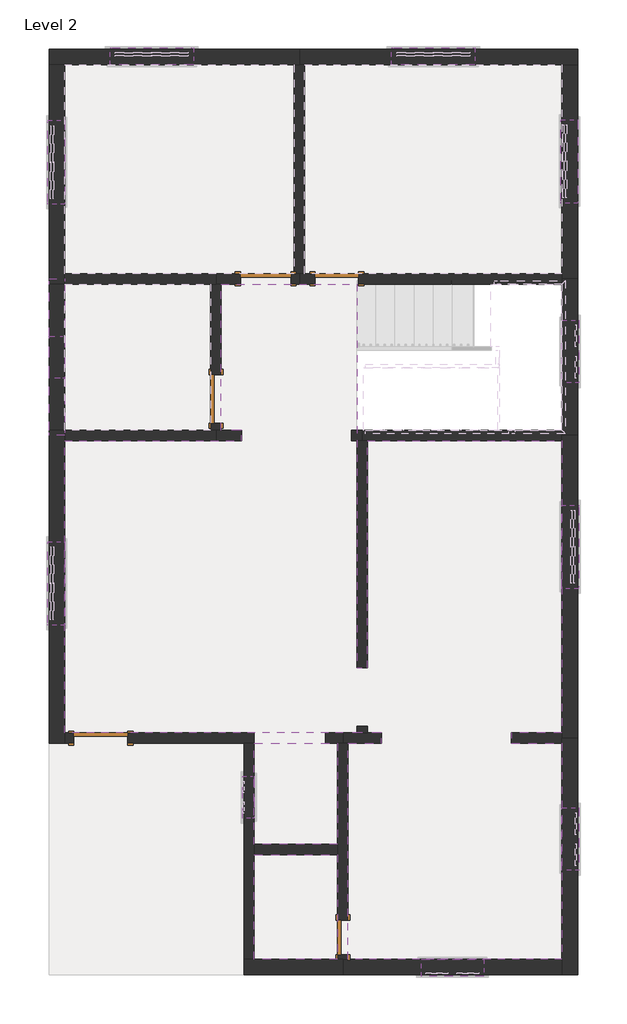
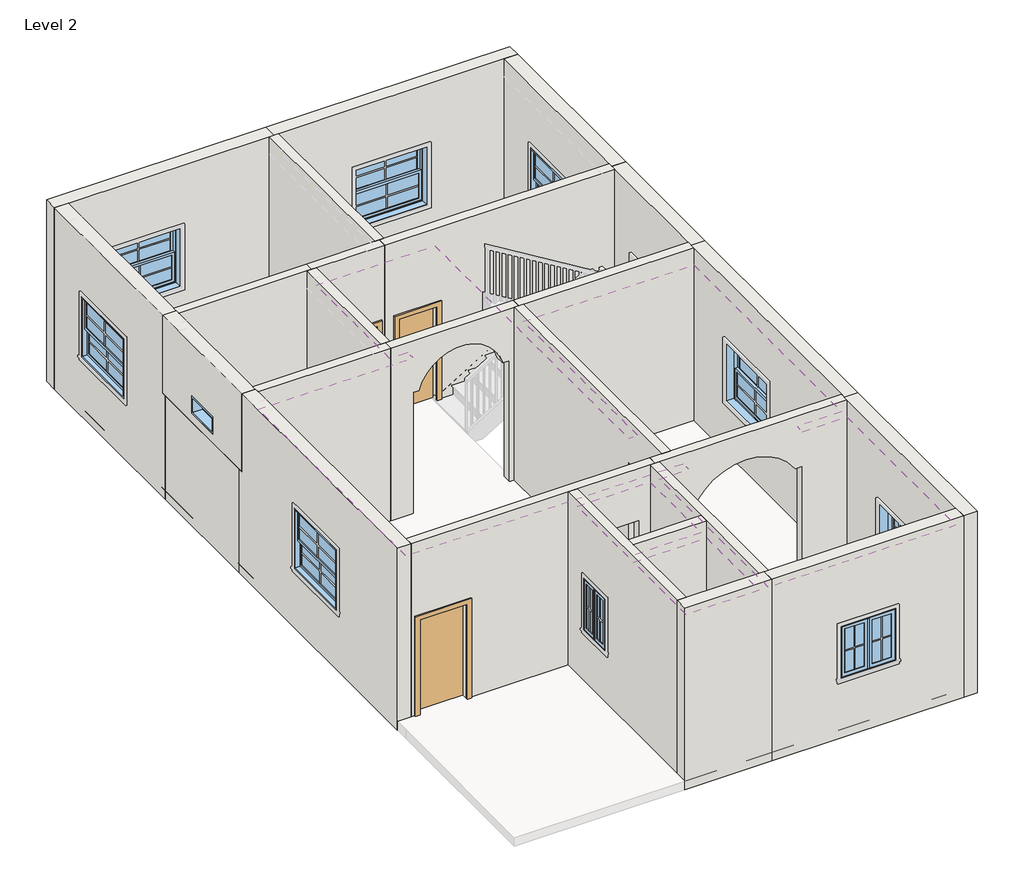
# One storey, part 1 of 2: 26 walls, 11 windows, 5 doors, 3 coverings.
"""IFC4 building model written with IfcOpenShell, lengths in millimetres."""

from ifc_helpers import new_model, si_unit, frame, origin, place, context, project, spatial, polyline, circle_curve, outline, extrude, faceted_brep, transform, mapped, element, save
from ifc_brep_helpers import plane_surface, revolved_surface, advanced_brep
from components import door_85c31a06, door_fe267433, door_77f51d0b, door_a6948854, door_ee35e093, fixed_2_8c8825d0, window_casement_double_2_fb285ced, window_casement_double_3_90de19e9, window_double_hung_4_eadb0177, window_double_hung_4_aab3aae7

model = new_model("IFC4")

# Units and contexts
model_context = context("Model", 3, world=origin())
ifc_project = project(units=[si_unit("LENGTHUNIT", "METRE", prefix="MILLI")], contexts=[model_context])

# Site, building, storey
site = spatial("IfcSite", under=ifc_project)
building = spatial("IfcBuilding", under=site)
storey = spatial("IfcBuildingStorey", under=building, Name="Level 2", Elevation=3200.4)

# Coverings
placement = place(None, origin())
element("IfcCovering", 1, ObjectType="2' x 4' ACT System", at=placement, inside=storey, context=model_context, shape_type="SweptSolid", body=[
    extrude(outline(polyline([(1592.635938, -3451.4142637), (1592.635938, -6601.0142637), (-1531.564062, -6601.0142637), (-1531.564062, -3451.4142637), (-1042.9877715, -3451.4142637), (-1042.9877715, -3299.0142637), (-1607.764062, -3299.0142637), (-5671.764062, -3299.0142637), (-5671.764062, 968.1857363), (-3538.164062, 968.1857363), (-3088.5741654, 968.1857363), (-3088.5741654, 1120.5857363), (-3385.764062, 1120.5857363), (-3385.764062, 3254.1857363), (-2242.764062, 3254.1857363), (-1404.564062, 3254.1857363), (-1404.564062, -2346.4297845), (-1252.164062, -2346.4297845), (-1252.164062, 968.1857363), (1592.635938, 968.1857363), (1592.635938, -3299.0142637), (852.655246, -3299.0142637), (852.655246, -3451.4142637), (1592.635938, -3451.4142637)])), frame((0.0, 0.0, 6248.4), z_axis=(0.0, 0.0, 1.0), x_axis=(1.0, 0.0, 0.0)), (0.0, 0.0, 1.0), 57.15),
])
element("IfcCovering", 2, ObjectType="2' x 4' ACT System", at=placement, inside=storey, context=model_context, shape_type="SweptSolid", body=[
    extrude(outline(polyline([(-2903.164062, -4924.6142637), (-2903.164062, -3451.4142637), (-1683.964062, -3451.4142637), (-1683.964062, -4924.6142637), (-2903.164062, -4924.6142637)])), frame((0.0, 0.0, 6248.4), z_axis=(0.0, 0.0, 1.0), x_axis=(1.0, 0.0, 0.0)), (0.0, 0.0, 1.0), 57.15),
])
element("IfcCovering", 3, ObjectType="2' x 4' ACT System", at=placement, inside=storey, context=model_context, shape_type="SweptSolid", body=[
    extrude(outline(polyline([(-2903.164062, -6601.0142637), (-2903.164062, -5077.0142637), (-1683.964062, -5077.0142637), (-1683.964062, -6601.0142637), (-2903.164062, -6601.0142637)])), frame((0.0, 0.0, 6248.4), z_axis=(0.0, 0.0, 1.0), x_axis=(1.0, 0.0, 0.0)), (0.0, 0.0, 1.0), 57.15),
])

# Doors
door_shape = door_85c31a06(model_context)
element("IfcDoor", 4, ObjectType="Single-Flush : 1'8\"", at=placement, inside=storey, context=model_context, shape_type="MappedRepresentation", body=[
    mapped(door_shape, transform((-1607.764062, -6283.5142637, 3352.8), x_axis=(0.0, -1.0, 0.0), y_axis=(1.0, 0.0, 0.0), z_axis=(0.0, 0.0, 1.0))),
])
door_2_shape = door_fe267433(model_context)
element("IfcDoor", 5, ObjectType="Single-Flush : 2'1\"", at=placement, inside=storey, context=model_context, shape_type="MappedRepresentation", body=[
    mapped(door_2_shape, transform((-1696.664062, 3330.3857363, 3352.8), x_axis=(-1.0, 0.0, 0.0), y_axis=(0.0, -1.0, 0.0), z_axis=(0.0, 0.0, 1.0))),
])
door_3_shape = door_77f51d0b(model_context)
element("IfcDoor", 6, ObjectType="Single-Flush : 2'4\"", at=placement, inside=storey, context=model_context, shape_type="MappedRepresentation", body=[
    mapped(door_3_shape, transform((-3461.964062, 1577.7857363, 3352.8), x_axis=(0.0, -1.0, 0.0), y_axis=(1.0, 0.0, 0.0), z_axis=(0.0, 0.0, 1.0))),
])
door_4_shape = door_a6948854(model_context)
element("IfcDoor", 7, ObjectType="Single-Flush : 2'5\"", at=placement, inside=storey, context=model_context, shape_type="MappedRepresentation", body=[
    mapped(door_4_shape, transform((-2738.064062, 3330.3857363, 3352.8), x_axis=(1.0, 0.0, 0.0), y_axis=(0.0, 1.0, 0.0), z_axis=(0.0, 0.0, 1.0))),
])
door_5_shape = door_ee35e093(model_context)
element("IfcDoor", 8, ObjectType="Single-Flush : 2'7\"", at=placement, inside=storey, context=model_context, shape_type="MappedRepresentation", body=[
    mapped(door_5_shape, transform((-5144.714062, -3375.2142637, 3352.8), x_axis=(-1.0, 0.0, 0.0), y_axis=(0.0, -1.0, 0.0), z_axis=(0.0, 0.0, 1.0))),
])

# Walls
element("IfcWall", 9, ObjectType="Generic - 6\"", at=placement, inside=storey, context=model_context, shape_type="Brep", body=[
    faceted_brep([(-2318.964062, 6454.5857363, 3352.8), (-2318.964062, 3406.5857363, 3352.8), (-2318.964062, 3406.5857363, 6553.2), (-2318.964062, 6454.5857363, 6553.2), (-2166.564062, 6454.5857363, 3352.8), (-2166.564062, 6454.5857363, 6553.2), (-2166.564062, 3406.5857363, 6553.2), (-2166.564062, 3406.5857363, 3352.8), (-2242.764062, 6454.5857363, 3352.8), (-2242.764062, 3406.5857363, 3352.8), (-2242.764062, 3406.5857363, 6553.2), (-2242.764062, 6454.5857363, 6553.2)], [[[0, 1, 2, 3]], [[4, 5, 6, 7]], [[1, 0, 8, 4, 7, 9]], [[3, 2, 10, 6, 5, 11]], [[0, 3, 11, 5, 4, 8]], [[2, 1, 9, 7, 6, 10]]]),
])
element("IfcWall", 10, ObjectType="Generic - 6\"", at=placement, inside=storey, context=model_context, shape_type="Brep", body=[
    faceted_brep([(-5671.764062, 3254.1857363, 6553.2), (-5671.764062, 3254.1857363, 5181.6), (-5671.764062, 3254.1857363, 3352.8), (-3538.164062, 3254.1857363, 3352.8), (-3461.964062, 3254.1857363, 3352.8), (-3461.964062, 3254.1857363, 6553.2), (-3538.164062, 3254.1857363, 6553.2), (-5671.764062, 3406.5857363, 3352.8), (-5671.764062, 3406.5857363, 6553.2), (-3461.964062, 3406.5857363, 6553.2), (-3461.964062, 3406.5857363, 3352.8), (-5671.764062, 3330.3857363, 6553.2)], [[[0, 1, 2, 3, 4, 5, 6]], [[7, 8, 9, 10]], [[4, 3, 2, 7, 10]], [[5, 4, 10, 9]], [[0, 6, 5, 9, 8, 11]], [[0, 11, 8, 7, 2, 1]]]),
])
element("IfcWall", 11, ObjectType="Generic - 6\"", at=placement, inside=storey, context=model_context, shape_type="Brep", body=[
    faceted_brep([(-5671.764062, 968.1857363, 6553.2), (-5671.764062, 968.1857363, 3352.8), (-3461.964062, 968.1857363, 3352.8), (-3461.964062, 968.1857363, 6553.2), (-5671.764062, 1120.5857363, 3352.8), (-5671.764062, 1120.5857363, 5181.6), (-5671.764062, 1120.5857363, 6553.2), (-3538.164062, 1120.5857363, 6553.2), (-3461.964062, 1120.5857363, 6553.2), (-3461.964062, 1120.5857363, 3352.8), (-3538.164062, 1120.5857363, 3352.8), (-5671.764062, 1044.3857363, 6553.2)], [[[0, 1, 2, 3]], [[4, 5, 6, 7, 8, 9, 10]], [[2, 1, 4, 10, 9]], [[3, 2, 9, 8]], [[0, 3, 8, 7, 6, 11]], [[0, 11, 6, 5, 4, 1]]]),
])
element("IfcWall", 12, ObjectType="Generic - 6\"", at=placement, inside=storey, context=model_context, shape_type="Brep", body=[
    faceted_brep([(-1404.564062, 968.1857363, 3352.8), (-1404.564062, -2346.4297845, 3352.8), (-1404.564062, -2346.4297845, 5816.6), (-1404.564062, -3197.4142637, 5816.6), (-1404.564062, -3197.4142637, 5638.8), (-1404.564062, -3197.4142637, 3352.8), (-1404.564062, -3299.0142637, 3352.8), (-1404.564062, -3299.0142637, 6553.2), (-1404.564062, 968.1857363, 6553.2), (-1252.164062, -2346.4297845, 3352.8), (-1252.164062, 968.1857363, 3352.8), (-1252.164062, 968.1857363, 6553.2), (-1252.164062, -3299.0142637, 6553.2), (-1252.164062, -3299.0142637, 3352.8), (-1252.164062, -3197.4142637, 3352.8), (-1252.164062, -3197.4142637, 5638.8), (-1252.164062, -3197.4142637, 5816.6), (-1252.164062, -2346.4297845, 5816.6), (-1328.364062, 968.1857363, 3352.8), (-1328.364062, 968.1857363, 6553.2)], [[[0, 1, 2, 3, 4, 5, 6, 7, 8]], [[9, 10, 11, 12, 13, 14, 15, 16, 17]], [[7, 6, 13, 12]], [[1, 0, 18, 10, 9]], [[8, 7, 12, 11, 19]], [[2, 1, 9, 17]], [[3, 2, 17, 16]], [[3, 16, 15, 14, 5, 4]], [[6, 5, 14, 13]], [[0, 8, 19, 11, 10, 18]]]),
])
element("IfcWall", 13, ObjectType="Generic - 6\"", at=placement, inside=storey, context=model_context, shape_type="Brep", body=[
    faceted_brep([(-2903.164062, -3451.4142637, 5638.8), (-1865.8319448, -3451.4142637, 5638.8), (-1865.8319448, -3451.4142637, 3352.8), (-1683.964062, -3451.4142637, 3352.8), (-1607.764062, -3451.4142637, 3352.8), (-1607.764062, -3451.4142637, 6553.2), (-1683.964062, -3451.4142637, 6553.2), (-2903.164062, -3451.4142637, 6553.2), (-3055.564062, -3451.4142637, 6553.2), (-5671.764062, -3451.4142637, 6553.2), (-5671.764062, -3451.4142637, 3352.8), (-5538.414062, -3451.4142637, 3352.8), (-5538.414062, -3451.4142637, 5181.6), (-4751.014062, -3451.4142637, 5181.6), (-4751.014062, -3451.4142637, 3352.8), (-3055.564062, -3451.4142637, 3352.8), (-2903.164062, -3451.4142637, 3352.8), (-1865.8319448, -3299.0142637, 5638.8), (-2903.164062, -3299.0142637, 5638.8), (-2903.164062, -3299.0142637, 3352.8), (-4751.014062, -3299.0142637, 3352.8), (-4751.014062, -3299.0142637, 5181.6), (-5538.414062, -3299.0142637, 5181.6), (-5538.414062, -3299.0142637, 3352.8), (-5671.764062, -3299.0142637, 3352.8), (-5671.764062, -3299.0142637, 6553.2), (-1607.764062, -3299.0142637, 6553.2), (-1607.764062, -3299.0142637, 3352.8), (-1865.8319448, -3299.0142637, 3352.8)], [[[0, 1, 2, 3, 4, 5, 6, 7, 8, 9, 10, 11, 12, 13, 14, 15, 16]], [[17, 18, 19, 20, 21, 22, 23, 24, 25, 26, 27, 28]], [[17, 1, 0, 18]], [[1, 17, 28, 2]], [[22, 12, 11, 23]], [[12, 22, 21, 13]], [[13, 21, 20, 14]], [[10, 24, 23, 11]], [[27, 4, 3, 2, 28]], [[19, 16, 15, 14, 20]], [[5, 4, 27, 26]], [[9, 8, 7, 6, 5, 26, 25]], [[10, 9, 25, 24]], [[18, 0, 16, 19]]]),
])
element("IfcWall", 14, ObjectType="Generic - 6\"", at=placement, inside=storey, context=model_context, shape_type="Brep", body=[
    faceted_brep([(-3055.564062, -3451.4142637, 3352.8), (-3055.564062, -6601.0142637, 3352.8), (-3055.564062, -6601.0142637, 6553.2), (-3055.564062, -3451.4142637, 6553.2), (-3055.564062, -3934.0142637, 5334.0), (-3055.564062, -4543.6142637, 5334.0), (-3055.564062, -4543.6142637, 4419.6), (-3055.564062, -3934.0142637, 4419.6), (-2903.164062, -3451.4142637, 3352.8), (-2903.164062, -3451.4142637, 5638.8), (-2903.164062, -3451.4142637, 6553.2), (-2903.164062, -4924.6142637, 6553.2), (-2903.164062, -5077.0142637, 6553.2), (-2903.164062, -6601.0142637, 6553.2), (-2903.164062, -6601.0142637, 3352.8), (-2903.164062, -5077.0142637, 3352.8), (-2903.164062, -4924.6142637, 3352.8), (-2903.164062, -3934.0142637, 5334.0), (-2903.164062, -3934.0142637, 4419.6), (-2903.164062, -4543.6142637, 4419.6), (-2903.164062, -4543.6142637, 5334.0)], [[[0, 1, 2, 3], [4, 5, 6, 7]], [[8, 9, 10, 11, 12, 13, 14, 15, 16], [17, 18, 19, 20]], [[1, 0, 8, 16, 15, 14]], [[3, 2, 13, 12, 11, 10]], [[2, 1, 14, 13]], [[18, 17, 4, 7]], [[19, 18, 7, 6]], [[20, 19, 6, 5]], [[17, 20, 5, 4]], [[0, 3, 10, 9, 8]]]),
])
element("IfcWall", 15, ObjectType="Generic - 6\"", at=placement, inside=storey, context=model_context, shape_type="Brep", body=[
    faceted_brep([(-1683.964062, -6601.0142637, 6553.2), (-1683.964062, -5077.0142637, 6553.2), (-1683.964062, -4924.6142637, 6553.2), (-1683.964062, -3451.4142637, 6553.2), (-1683.964062, -3451.4142637, 3352.8), (-1683.964062, -4924.6142637, 3352.8), (-1683.964062, -5077.0142637, 3352.8), (-1683.964062, -6029.5142637, 3352.8), (-1683.964062, -6029.5142637, 5181.6), (-1683.964062, -6537.5142637, 5181.6), (-1683.964062, -6537.5142637, 3352.8), (-1683.964062, -6601.0142637, 3352.8), (-1531.564062, -3451.4142637, 6553.2), (-1531.564062, -6601.0142637, 6553.2), (-1531.564062, -6601.0142637, 3352.8), (-1531.564062, -6537.5142637, 3352.8), (-1531.564062, -6537.5142637, 5181.6), (-1531.564062, -6029.5142637, 5181.6), (-1531.564062, -6029.5142637, 3352.8), (-1531.564062, -3451.4142637, 3352.8), (-1607.764062, -6601.0142637, 3352.8), (-1607.764062, -3451.4142637, 3352.8), (-1607.764062, -6601.0142637, 6553.2), (-1607.764062, -3451.4142637, 6553.2)], [[[0, 1, 2, 3, 4, 5, 6, 7, 8, 9, 10, 11]], [[12, 13, 14, 15, 16, 17, 18, 19]], [[14, 20, 11, 10, 15]], [[4, 21, 19, 18, 7, 6, 5]], [[3, 2, 1, 0, 22, 13, 12, 23]], [[9, 16, 15, 10]], [[16, 9, 8, 17]], [[17, 8, 7, 18]], [[0, 11, 20, 14, 13, 22]], [[4, 3, 23, 12, 19, 21]]]),
])
element("IfcWall", 16, ObjectType="Generic - 6\"", at=placement, inside=storey, context=model_context, shape_type="SweptSolid", body=[
    extrude(outline(polyline([(-1683.964062, -5077.0142637), (-2903.164062, -5077.0142637), (-2903.164062, -4924.6142637), (-1683.964062, -4924.6142637), (-1683.964062, -5077.0142637)])), frame((0.0, 0.0, 3352.8), z_axis=(0.0, 0.0, 1.0), x_axis=(1.0, 0.0, 0.0)), (0.0, 0.0, 1.0), 3200.4),
])
element("IfcWall", 17, ObjectType="Generic - 6\"", at=placement, inside=storey, context=model_context, shape_type="Brep", body=[
    faceted_brep([(-3538.164062, 1120.5857363, 6553.2), (-3538.164062, 3254.1857363, 6553.2), (-3538.164062, 3254.1857363, 3352.8), (-3538.164062, 1933.3857363, 3352.8), (-3538.164062, 1933.3857363, 5181.6), (-3538.164062, 1222.1857363, 5181.6), (-3538.164062, 1222.1857363, 3352.8), (-3538.164062, 1120.5857363, 3352.8), (-3385.764062, 3254.1857363, 6553.2), (-3385.764062, 1120.5857363, 6553.2), (-3385.764062, 1120.5857363, 3352.8), (-3385.764062, 1222.1857363, 3352.8), (-3385.764062, 1222.1857363, 5181.6), (-3385.764062, 1933.3857363, 5181.6), (-3385.764062, 1933.3857363, 3352.8), (-3385.764062, 3254.1857363, 3352.8), (-3461.964062, 3254.1857363, 3352.8), (-3461.964062, 1120.5857363, 3352.8), (-3461.964062, 1120.5857363, 6553.2), (-3461.964062, 3254.1857363, 6553.2)], [[[0, 1, 2, 3, 4, 5, 6, 7]], [[8, 9, 10, 11, 12, 13, 14, 15]], [[2, 16, 15, 14, 3]], [[10, 17, 7, 6, 11]], [[1, 0, 18, 9, 8, 19]], [[12, 5, 4, 13]], [[13, 4, 3, 14]], [[5, 12, 11, 6]], [[2, 1, 19, 8, 15, 16]], [[0, 7, 17, 10, 9, 18]]]),
])
element("IfcWall", 18, ObjectType="Generic - 6\"", at=placement, inside=storey, context=model_context, shape_type="Brep", body=[
    faceted_brep([(-2242.764062, 3254.1857363, 3352.8), (-2014.164062, 3254.1857363, 3352.8), (-2014.164062, 3254.1857363, 5181.6), (-1379.164062, 3254.1857363, 5181.6), (-1379.164062, 3254.1857363, 3352.8), (1592.635938, 3254.1857363, 3352.8), (1592.635938, 3254.1857363, 6553.2), (-2242.764062, 3254.1857363, 6553.2), (-2014.164062, 3406.5857363, 5181.6), (-2014.164062, 3406.5857363, 3352.8), (-2166.564062, 3406.5857363, 3352.8), (-2242.764062, 3406.5857363, 3352.8), (-2242.764062, 3406.5857363, 6553.2), (-2166.564062, 3406.5857363, 6553.2), (1592.635938, 3406.5857363, 6553.2), (1592.635938, 3406.5857363, 3352.8), (-1379.164062, 3406.5857363, 3352.8), (-1379.164062, 3406.5857363, 5181.6), (1592.635938, 3330.3857363, 3352.8), (1592.635938, 3330.3857363, 6553.2)], [[[0, 1, 2, 3, 4, 5, 6, 7]], [[8, 9, 10, 11, 12, 13, 14, 15, 16, 17]], [[16, 15, 18, 5, 4]], [[11, 10, 9, 1, 0]], [[7, 6, 19, 14, 13, 12]], [[0, 7, 12, 11]], [[6, 5, 18, 15, 14, 19]], [[4, 3, 17, 16]], [[3, 2, 8, 17]], [[2, 1, 9, 8]]]),
])
element("IfcWall", 19, ObjectType="Generic - 6\"", at=placement, inside=storey, context=model_context, shape_type="Brep", body=[
    faceted_brep([(1592.635938, 968.1857363, 6553.2), (-1252.164062, 968.1857363, 6553.2), (-1328.364062, 968.1857363, 6553.2), (-1328.364062, 968.1857363, 3352.8), (-1252.164062, 968.1857363, 3352.8), (1592.635938, 968.1857363, 3352.8), (1592.635938, 1120.5857363, 6553.2), (1592.635938, 1120.5857363, 3352.8), (-1328.364062, 1120.5857363, 3352.8), (-1328.364062, 1120.5857363, 6553.2), (1592.635938, 1044.3857363, 6553.2), (1592.635938, 1044.3857363, 3352.8)], [[[0, 1, 2, 3, 4, 5]], [[6, 7, 8, 9]], [[2, 1, 0, 10, 6, 9]], [[5, 4, 3, 8, 7, 11]], [[2, 9, 8, 3]], [[0, 5, 11, 7, 6, 10]]]),
])
element("IfcWall", 20, ObjectType="Generic - 6\"", at=placement, inside=storey, context=model_context, shape_type="AdvancedBrep", body=[
    advanced_brep(
    [(1592.635938, -3451.4142637, 6553.2), (-1531.564062, -3451.4142637, 6553.2), (-1607.764062, -3451.4142637, 6553.2), (-1607.764062, -3451.4142637, 3352.8), (-1531.564062, -3451.4142637, 3352.8), (-1042.9877715, -3451.4142637, 3352.8), (-1042.9877715, -3451.4142637, 5638.8), (-909.3649468, -3451.4142637, 5638.8), (732.5205767, -3451.4142637, 5638.8), (852.655246, -3451.4142637, 5638.8), (852.655246, -3451.4142637, 3352.8), (1592.635938, -3451.4142637, 3352.8), (-1607.764062, -3299.0142637, 6553.2), (-1404.564062, -3299.0142637, 6553.2), (-1252.164062, -3299.0142637, 6553.2), (1592.635938, -3299.0142637, 6553.2), (1592.635938, -3299.0142637, 3352.8), (852.655246, -3299.0142637, 3352.8), (852.655246, -3299.0142637, 5638.8), (732.5205767, -3299.0142637, 5638.8), (-909.3649468, -3299.0142637, 5638.8), (-1042.9877715, -3299.0142637, 5638.8), (-1042.9877715, -3299.0142637, 3352.8), (-1252.164062, -3299.0142637, 3352.8), (-1404.564062, -3299.0142637, 3352.8), (-1607.764062, -3299.0142637, 3352.8), (1592.635938, -3375.2142637, 6553.2), (1592.635938, -3375.2142637, 3352.8)],
    [
        (0, 1),
        (1, 2),
        (2, 3),
        (3, 4),
        (4, 5),
        (5, 6),
        (6, 7),
        (7, 8, circle_curve(frame((-88.4221851, -3451.4142637, 5103.0141821), z_axis=(0.0, 1.0, 0.0), x_axis=(-1.0, 0.0, 0.0)), 980.3129402)),
        (8, 9),
        (9, 10),
        (10, 11),
        (11, 0),
        (12, 13),
        (13, 14),
        (14, 15),
        (15, 16),
        (16, 17),
        (17, 18),
        (18, 19),
        (19, 20, circle_curve(frame((-88.4221851, -3299.0142637, 5103.0141821), z_axis=(0.0, -1.0, 0.0), x_axis=(-1.0, 0.0, 0.0)), 980.3129402)),
        (20, 21),
        (21, 22),
        (22, 23),
        (23, 24),
        (24, 25),
        (25, 12),
        (0, 26),
        (26, 15),
        (12, 2),
        (9, 18),
        (17, 10),
        (5, 22),
        (21, 6),
        (7, 20),
        (19, 8),
        (3, 25),
        (16, 27),
        (27, 11),
    ],
    [
        plane_surface(frame((1706.935938, -3451.4142637, 6553.2), z_axis=(0.0, -1.0, 0.0), x_axis=(-1.0, 0.0, 0.0))),
        plane_surface(frame((1706.935938, -3299.0142637, 6553.2), z_axis=(0.0, 1.0, 0.0), x_axis=(1.0, 0.0, 0.0))),
        plane_surface(frame((1706.935938, -3451.4142637, 6553.2), z_axis=(0.0, 0.0, 1.0), x_axis=(0.0, 1.0, 0.0))),
        plane_surface(frame((852.655246, -3451.4142637, 5377.580621), z_axis=(-1.0, 0.0, 0.0), x_axis=(0.0, 1.0, 0.0))),
        plane_surface(frame((-1042.9877715, -3451.4142637, 3688.3784957), z_axis=(1.0, 0.0, 0.0), x_axis=(0.0, 1.0, 0.0))),
        revolved_surface(polyline([(-1068.7351253, -3299.0142637, 5103.0141821), (-1068.7351253, -3451.4142637, 5103.0141821)]), (-88.4221851, -3299.0142637, 5103.0141821), (0.0, 1.0, 0.0)),
        plane_surface(frame((-1607.764062, -3451.4142637, 3352.8), z_axis=(0.0, 0.0, -1.0), x_axis=(0.0, 1.0, 0.0))),
        plane_surface(frame((456.9071606, -3451.4142637, 3352.8), z_axis=(0.0, 0.0, -1.0), x_axis=(0.0, 1.0, 0.0))),
        plane_surface(frame((-1607.764062, -3451.4142637, 6553.2), z_axis=(-1.0, 0.0, 0.0), x_axis=(0.0, 1.0, 0.0))),
        plane_surface(frame((1592.635938, 6454.5857363, 3352.8), z_axis=(1.0, 0.0, 0.0), x_axis=(0.0, -1.0, 0.0))),
        plane_surface(frame((-1042.9877715, -3299.0142637, 5638.8), z_axis=(0.0, 0.0, -1.0), x_axis=(-1.0, 0.0, 0.0))),
    ],
    [
        (0, [[1, 2, 3, 4, 5, 6, 7, 8, 9, 10, 11, 12]]),
        (1, [[13, 14, 15, 16, 17, 18, 19, 20, 21, 22, 23, 24, 25, 26]]),
        (2, [[-2, -1, 27, 28, -15, -14, -13, 29]]),
        (3, [[30, -18, 31, -10]]),
        (4, [[32, -22, 33, -6]]),
        (5, [[-8, 34, -20, 35]]),
        (6, [[36, -25, -24, -23, -32, -5, -4]]),
        (7, [[37, 38, -11, -31, -17]]),
        (8, [[-3, -29, -26, -36]]),
        (9, [[-12, -38, -37, -16, -28, -27]]),
        (10, [[-33, -21, -34, -7]]),
        (10, [[-30, -9, -35, -19]]),
    ],
),
])
element("IfcWall", 21, ObjectType="Generic - 6\"", at=placement, inside=storey, context=model_context, shape_type="Brep", body=[
    faceted_brep([(-2369.764062, 3254.1857363, 5181.6), (-2369.764062, 3254.1857363, 3352.8), (-2242.764062, 3254.1857363, 3352.8), (-2242.764062, 3254.1857363, 6553.2), (-3385.764062, 3254.1857363, 6553.2), (-3461.964062, 3254.1857363, 6553.2), (-3461.964062, 3254.1857363, 3352.8), (-3385.764062, 3254.1857363, 3352.8), (-3106.364062, 3254.1857363, 3352.8), (-3106.364062, 3254.1857363, 5181.6), (-2242.764062, 3406.5857363, 3352.8), (-2318.964062, 3406.5857363, 3352.8), (-2369.764062, 3406.5857363, 3352.8), (-2369.764062, 3406.5857363, 5181.6), (-3106.364062, 3406.5857363, 5181.6), (-3106.364062, 3406.5857363, 3352.8), (-3461.964062, 3406.5857363, 3352.8), (-3461.964062, 3406.5857363, 6553.2), (-2318.964062, 3406.5857363, 6553.2), (-2242.764062, 3406.5857363, 6553.2)], [[[0, 1, 2, 3, 4, 5, 6, 7, 8, 9]], [[10, 11, 12, 13, 14, 15, 16, 17, 18, 19]], [[2, 1, 12, 11, 10]], [[8, 7, 6, 16, 15]], [[3, 2, 10, 19]], [[5, 4, 3, 19, 18, 17]], [[6, 5, 17, 16]], [[15, 14, 9, 8]], [[14, 13, 0, 9]], [[13, 12, 1, 0]]]),
])
element("IfcWall", 22, ObjectType="Generic - 6\"", at=placement, inside=storey, context=model_context, shape_type="AdvancedBrep", body=[
    advanced_brep(
    [(-1328.364062, 968.1857363, 6553.2), (-1404.564062, 968.1857363, 6553.2), (-3461.964062, 968.1857363, 6553.2), (-3461.964062, 968.1857363, 3352.8), (-3088.5741654, 968.1857363, 3352.8), (-3088.5741654, 968.1857363, 5638.8), (-2990.069581, 968.1857363, 5638.8), (-1595.0493956, 968.1857363, 5638.8), (-1480.764062, 968.1857363, 5638.8), (-1480.764062, 968.1857363, 3352.8), (-1404.564062, 968.1857363, 3352.8), (-1328.364062, 968.1857363, 3352.8), (-3461.964062, 1120.5857363, 6553.2), (-3385.764062, 1120.5857363, 6553.2), (-1328.364062, 1120.5857363, 6553.2), (-1328.364062, 1120.5857363, 3352.8), (-1480.764062, 1120.5857363, 3352.8), (-1480.764062, 1120.5857363, 5638.8), (-1595.0493956, 1120.5857363, 5638.8), (-2990.069581, 1120.5857363, 5638.8), (-3088.5741654, 1120.5857363, 5638.8), (-3088.5741654, 1120.5857363, 3352.8), (-3385.764062, 1120.5857363, 3352.8), (-3461.964062, 1120.5857363, 3352.8)],
    [
        (0, 1),
        (1, 2),
        (2, 3),
        (3, 4),
        (4, 5),
        (5, 6),
        (6, 7, circle_curve(frame((-2292.5594883, 968.1857363, 5461.0), z_axis=(0.0, 1.0, 0.0), x_axis=(-1.0, 0.0, 0.0)), 719.8146771)),
        (7, 8),
        (8, 9),
        (9, 10),
        (10, 11),
        (11, 0),
        (12, 13),
        (13, 14),
        (14, 15),
        (15, 16),
        (16, 17),
        (17, 18),
        (18, 19, circle_curve(frame((-2292.5594883, 1120.5857363, 5461.0), z_axis=(0.0, -1.0, 0.0), x_axis=(-1.0, 0.0, 0.0)), 719.8146771)),
        (19, 20),
        (20, 21),
        (21, 22),
        (22, 23),
        (23, 12),
        (6, 19),
        (18, 7),
        (15, 11),
        (9, 16),
        (0, 14),
        (12, 2),
        (3, 23),
        (21, 4),
        (5, 20),
        (17, 8),
    ],
    [
        plane_surface(frame((-3012.3741654, 968.1857363, 5461.0), z_axis=(0.0, -1.0, 0.0), x_axis=(0.0, 0.0, 1.0))),
        plane_surface(frame((-3012.3741654, 1120.5857363, 5461.0), z_axis=(0.0, 1.0, 0.0), x_axis=(0.0, 0.0, -1.0))),
        revolved_surface(polyline([(-3012.3741654, 1120.5857363, 5461.0), (-3012.3741654, 968.1857363, 5461.0)]), (-2292.5594883, 1120.5857363, 5461.0), (0.0, 1.0, 0.0)),
        plane_surface(frame((-1572.7448112, 968.1857363, 3352.8), z_axis=(0.0, 0.0, -1.0), x_axis=(0.0, 1.0, 0.0))),
        plane_surface(frame((-1328.364062, 968.1857363, 6553.2), z_axis=(0.0, 0.0, 1.0), x_axis=(0.0, 1.0, 0.0))),
        plane_surface(frame((-3461.964062, 968.1857363, 3352.8), z_axis=(0.0, 0.0, -1.0), x_axis=(0.0, 1.0, 0.0))),
        plane_surface(frame((-1328.364062, 968.1857363, 3352.8), z_axis=(1.0, 0.0, 0.0), x_axis=(0.0, 1.0, 0.0))),
        plane_surface(frame((-3461.964062, 968.1857363, 6553.2), z_axis=(-1.0, 0.0, 0.0), x_axis=(0.0, 1.0, 0.0))),
        plane_surface(frame((-3088.5741654, 1120.5857363, 5638.8), z_axis=(0.0, 0.0, -1.0), x_axis=(-1.0, 0.0, 0.0))),
        plane_surface(frame((-3088.5741654, 1120.5857363, 5638.8), z_axis=(1.0, 0.0, 0.0), x_axis=(0.0, 0.0, -1.0))),
        plane_surface(frame((-1480.764062, 968.1857363, 5638.8), z_axis=(-1.0, 0.0, 0.0), x_axis=(0.0, 0.0, -1.0))),
    ],
    [
        (0, [[1, 2, 3, 4, 5, 6, 7, 8, 9, 10, 11, 12]]),
        (1, [[13, 14, 15, 16, 17, 18, 19, 20, 21, 22, 23, 24]]),
        (2, [[-7, 25, -19, 26]]),
        (3, [[27, -11, -10, 28, -16]]),
        (4, [[-2, -1, 29, -14, -13, 30]]),
        (5, [[31, -23, -22, 32, -4]]),
        (6, [[-12, -27, -15, -29]]),
        (7, [[-3, -30, -24, -31]]),
        (8, [[33, -20, -25, -6]]),
        (8, [[34, -8, -26, -18]]),
        (9, [[-33, -5, -32, -21]]),
        (10, [[-34, -17, -28, -9]]),
    ],
),
])
element("IfcWall", 23, ObjectType="Generic - 9\"", at=placement, inside=storey, context=model_context, shape_type="Brep", body=[
    faceted_brep([(-5900.364062, 6454.5857363, 3352.8), (-5671.764062, 6454.5857363, 3352.8), (-2318.964062, 6454.5857363, 3352.8), (-2242.764062, 6454.5857363, 3352.8), (-2242.764062, 6454.5857363, 6553.2), (-2318.964062, 6454.5857363, 6553.2), (-5671.764062, 6454.5857363, 6553.2), (-5900.364062, 6454.5857363, 6553.2), (-3792.164062, 6454.5857363, 5486.4), (-3792.164062, 6454.5857363, 4419.6), (-5011.364062, 6454.5857363, 4419.6), (-5011.364062, 6454.5857363, 5486.4), (-5900.364062, 6683.1857363, 3352.8), (-5900.364062, 6683.1857363, 6553.2), (-2242.764062, 6683.1857363, 6553.2), (-2242.764062, 6683.1857363, 3352.8), (-3792.164062, 6683.1857363, 5486.4), (-5011.364062, 6683.1857363, 5486.4), (-5011.364062, 6683.1857363, 4419.6), (-3792.164062, 6683.1857363, 4419.6)], [[[0, 1, 2, 3, 4, 5, 6, 7], [8, 9, 10, 11]], [[12, 13, 14, 15], [16, 17, 18, 19]], [[3, 2, 1, 0, 12, 15]], [[4, 3, 15, 14]], [[7, 6, 5, 4, 14, 13]], [[0, 7, 13, 12]], [[9, 8, 16, 19]], [[10, 9, 19, 18]], [[11, 10, 18, 17]], [[8, 11, 17, 16]]]),
])
element("IfcWall", 24, ObjectType="Generic - 9\"", at=placement, inside=storey, context=model_context, shape_type="Brep", body=[
    faceted_brep([(1592.635938, 6454.5857363, 3352.8), (1592.635938, 3406.5857363, 3352.8), (1592.635938, 3330.3857363, 3352.8), (1592.635938, 3330.3857363, 6553.2), (1592.635938, 3406.5857363, 6553.2), (1592.635938, 6454.5857363, 6553.2), (1592.635938, 5654.4857363, 5486.4), (1592.635938, 4435.2857363, 5486.4), (1592.635938, 4435.2857363, 4419.6), (1592.635938, 5654.4857363, 4419.6), (1821.235938, 6454.5857363, 3352.8), (1821.235938, 6454.5857363, 6553.2), (1821.235938, 3330.3857363, 6553.2), (1821.235938, 3330.3857363, 3352.8), (1821.235938, 5654.4857363, 5486.4), (1821.235938, 5654.4857363, 4419.6), (1821.235938, 4435.2857363, 4419.6), (1821.235938, 4435.2857363, 5486.4)], [[[0, 1, 2, 3, 4, 5], [6, 7, 8, 9]], [[10, 11, 12, 13], [14, 15, 16, 17]], [[2, 1, 0, 10, 13]], [[3, 2, 13, 12]], [[5, 4, 3, 12, 11]], [[0, 5, 11, 10]], [[15, 14, 6, 9]], [[16, 15, 9, 8]], [[17, 16, 8, 7]], [[14, 17, 7, 6]]]),
])
element("IfcWall", 25, ObjectType="Generic - 9\"", at=placement, inside=storey, context=model_context, shape_type="Brep", body=[
    faceted_brep([(1592.635938, -6601.0142637, 3352.8), (-1531.564062, -6601.0142637, 3352.8), (-1607.764062, -6601.0142637, 3352.8), (-1607.764062, -6601.0142637, 6553.2), (-1531.564062, -6601.0142637, 6553.2), (1592.635938, -6601.0142637, 6553.2), (-464.764062, -6601.0142637, 5334.0), (-464.764062, -6601.0142637, 4419.6), (449.635938, -6601.0142637, 4419.6), (449.635938, -6601.0142637, 5334.0), (1592.635938, -6829.6142637, 3352.8), (1592.635938, -6829.6142637, 6553.2), (-1607.764062, -6829.6142637, 6553.2), (-1607.764062, -6829.6142637, 3352.8), (-464.764062, -6829.6142637, 5334.0), (449.635938, -6829.6142637, 5334.0), (449.635938, -6829.6142637, 4419.6), (-464.764062, -6829.6142637, 4419.6)], [[[0, 1, 2, 3, 4, 5], [6, 7, 8, 9]], [[10, 11, 12, 13], [14, 15, 16, 17]], [[2, 1, 0, 10, 13]], [[3, 2, 13, 12]], [[5, 4, 3, 12, 11]], [[0, 5, 11, 10]], [[7, 6, 14, 17]], [[8, 7, 17, 16]], [[9, 8, 16, 15]], [[6, 9, 15, 14]]]),
])
element("IfcWall", 26, ObjectType="Generic - 9\"", at=placement, inside=storey, context=model_context, shape_type="Brep", body=[
    faceted_brep([(-5900.364062, 6454.5857363, 3352.8), (-5900.364062, 3254.1857363, 3352.8), (-5900.364062, 3254.1857363, 5181.6), (-5900.364062, 3330.3857363, 5181.6), (-5900.364062, 3330.3857363, 6553.2), (-5900.364062, 6454.5857363, 6553.2), (-5900.364062, 4422.5857363, 5486.4), (-5900.364062, 4422.5857363, 4419.6), (-5900.364062, 5641.7857363, 4419.6), (-5900.364062, 5641.7857363, 5486.4), (-5671.764062, 6454.5857363, 3352.8), (-5671.764062, 6454.5857363, 6553.2), (-5671.764062, 3406.5857363, 6553.2), (-5671.764062, 3330.3857363, 6553.2), (-5671.764062, 3330.3857363, 5181.6), (-5671.764062, 3254.1857363, 5181.6), (-5671.764062, 3254.1857363, 3352.8), (-5671.764062, 3406.5857363, 3352.8), (-5671.764062, 4422.5857363, 5486.4), (-5671.764062, 5641.7857363, 5486.4), (-5671.764062, 5641.7857363, 4419.6), (-5671.764062, 4422.5857363, 4419.6)], [[[0, 1, 2, 3, 4, 5], [6, 7, 8, 9]], [[10, 11, 12, 13, 14, 15, 16, 17], [18, 19, 20, 21]], [[1, 0, 10, 17, 16]], [[5, 4, 13, 12, 11]], [[0, 5, 11, 10]], [[7, 6, 18, 21]], [[8, 7, 21, 20]], [[9, 8, 20, 19]], [[6, 9, 19, 18]], [[4, 3, 14, 13]], [[14, 3, 2, 15]], [[2, 1, 16, 15]]]),
])
element("IfcWall", 27, ObjectType="Generic - 9\"", at=placement, inside=storey, context=model_context, shape_type="Brep", body=[
    faceted_brep([(-2242.764062, 6454.5857363, 3352.8), (-2166.564062, 6454.5857363, 3352.8), (1592.635938, 6454.5857363, 3352.8), (1821.235938, 6454.5857363, 3352.8), (1821.235938, 6454.5857363, 6553.2), (1592.635938, 6454.5857363, 6553.2), (-2166.564062, 6454.5857363, 6553.2), (-2242.764062, 6454.5857363, 6553.2), (322.635938, 6454.5857363, 5486.4), (322.635938, 6454.5857363, 4419.6), (-896.564062, 6454.5857363, 4419.6), (-896.564062, 6454.5857363, 5486.4), (-2242.764062, 6683.1857363, 3352.8), (-2242.764062, 6683.1857363, 6553.2), (1821.235938, 6683.1857363, 6553.2), (1821.235938, 6683.1857363, 3352.8), (322.635938, 6683.1857363, 5486.4), (-896.564062, 6683.1857363, 5486.4), (-896.564062, 6683.1857363, 4419.6), (322.635938, 6683.1857363, 4419.6)], [[[0, 1, 2, 3, 4, 5, 6, 7], [8, 9, 10, 11]], [[12, 13, 14, 15], [16, 17, 18, 19]], [[3, 2, 1, 0, 12, 15]], [[7, 6, 5, 4, 14, 13]], [[0, 7, 13, 12]], [[4, 3, 15, 14]], [[8, 11, 17, 16]], [[11, 10, 18, 17]], [[10, 9, 19, 18]], [[9, 8, 16, 19]]]),
])
element("IfcWall", 28, ObjectType="Generic - 9\"", at=placement, inside=storey, context=model_context, shape_type="Brep", body=[
    faceted_brep([(-1607.764062, -6601.0142637, 3352.8), (-1683.964062, -6601.0142637, 3352.8), (-2903.164062, -6601.0142637, 3352.8), (-3055.564062, -6601.0142637, 3352.8), (-3055.564062, -6601.0142637, 6553.2), (-2903.164062, -6601.0142637, 6553.2), (-1683.964062, -6601.0142637, 6553.2), (-1607.764062, -6601.0142637, 6553.2), (-1607.764062, -6829.6142637, 3352.8), (-1607.764062, -6829.6142637, 6553.2), (-3055.564062, -6829.6142637, 6553.2), (-3055.564062, -6829.6142637, 3352.8)], [[[0, 1, 2, 3, 4, 5, 6, 7]], [[8, 9, 10, 11]], [[3, 2, 1, 0, 8, 11]], [[7, 6, 5, 4, 10, 9]], [[0, 7, 9, 8]], [[4, 3, 11, 10]]]),
])
element("IfcWall", 29, ObjectType="Generic - 9\"", at=placement, inside=storey, context=model_context, shape_type="Brep", body=[
    faceted_brep([(1592.635938, 3330.3857363, 3352.8), (1592.635938, 3254.1857363, 3352.8), (1592.635938, 1120.5857363, 3352.8), (1592.635938, 1044.3857363, 3352.8), (1592.635938, 1044.3857363, 6553.2), (1592.635938, 1120.5857363, 6553.2), (1592.635938, 3254.1857363, 6553.2), (1592.635938, 3330.3857363, 6553.2), (1592.635938, 1812.7357363, 5334.0), (1592.635938, 1812.7357363, 4419.6), (1592.635938, 2727.1357363, 4419.6), (1592.635938, 2727.1357363, 5334.0), (1821.235938, 3330.3857363, 3352.8), (1821.235938, 3330.3857363, 6553.2), (1821.235938, 1044.3857363, 6553.2), (1821.235938, 1044.3857363, 3352.8), (1821.235938, 1812.7357363, 5334.0), (1821.235938, 2727.1357363, 5334.0), (1821.235938, 2727.1357363, 4419.6), (1821.235938, 1812.7357363, 4419.6)], [[[0, 1, 2, 3, 4, 5, 6, 7], [8, 9, 10, 11]], [[12, 13, 14, 15], [16, 17, 18, 19]], [[3, 2, 1, 0, 12, 15]], [[4, 3, 15, 14]], [[7, 6, 5, 4, 14, 13]], [[0, 7, 13, 12]], [[8, 11, 17, 16]], [[11, 10, 18, 17]], [[10, 9, 19, 18]], [[9, 8, 16, 19]]]),
])
element("IfcWall", 30, ObjectType="Generic - 9\"", at=placement, inside=storey, context=model_context, shape_type="Brep", body=[
    faceted_brep([(1592.635938, 1044.3857363, 3352.8), (1592.635938, 968.1857363, 3352.8), (1592.635938, -3299.0142637, 3352.8), (1592.635938, -3375.2142637, 3352.8), (1592.635938, -3375.2142637, 6553.2), (1592.635938, -3299.0142637, 6553.2), (1592.635938, 968.1857363, 6553.2), (1592.635938, 1044.3857363, 6553.2), (1592.635938, 28.3857363, 5486.4), (1592.635938, -1190.8142637, 5486.4), (1592.635938, -1190.8142637, 4419.6), (1592.635938, 28.3857363, 4419.6), (1821.235938, 1044.3857363, 3352.8), (1821.235938, 1044.3857363, 6553.2), (1821.235938, -3375.2142637, 6553.2), (1821.235938, -3375.2142637, 3352.8), (1821.235938, 28.3857363, 5486.4), (1821.235938, 28.3857363, 4419.6), (1821.235938, -1190.8142637, 4419.6), (1821.235938, -1190.8142637, 5486.4)], [[[0, 1, 2, 3, 4, 5, 6, 7], [8, 9, 10, 11]], [[12, 13, 14, 15], [16, 17, 18, 19]], [[3, 2, 1, 0, 12, 15]], [[4, 3, 15, 14]], [[7, 6, 5, 4, 14, 13]], [[0, 7, 13, 12]], [[16, 19, 9, 8]], [[19, 18, 10, 9]], [[18, 17, 11, 10]], [[17, 16, 8, 11]]]),
])
element("IfcWall", 31, ObjectType="Generic - 9\"", at=placement, inside=storey, context=model_context, shape_type="Brep", body=[
    faceted_brep([(1592.635938, -3375.2142637, 3352.8), (1592.635938, -3451.4142637, 3352.8), (1592.635938, -6601.0142637, 3352.8), (1592.635938, -6829.6142637, 3352.8), (1592.635938, -6829.6142637, 6553.2), (1592.635938, -6601.0142637, 6553.2), (1592.635938, -3451.4142637, 6553.2), (1592.635938, -3375.2142637, 6553.2), (1592.635938, -5305.6142637, 5334.0), (1592.635938, -5305.6142637, 4419.6), (1592.635938, -4391.2142637, 4419.6), (1592.635938, -4391.2142637, 5334.0), (1821.235938, -3375.2142637, 3352.8), (1821.235938, -3375.2142637, 6553.2), (1821.235938, -6829.6142637, 6553.2), (1821.235938, -6829.6142637, 3352.8), (1821.235938, -5305.6142637, 5334.0), (1821.235938, -4391.2142637, 5334.0), (1821.235938, -4391.2142637, 4419.6), (1821.235938, -5305.6142637, 4419.6)], [[[0, 1, 2, 3, 4, 5, 6, 7], [8, 9, 10, 11]], [[12, 13, 14, 15], [16, 17, 18, 19]], [[3, 2, 1, 0, 12, 15]], [[7, 6, 5, 4, 14, 13]], [[0, 7, 13, 12]], [[4, 3, 15, 14]], [[8, 11, 17, 16]], [[11, 10, 18, 17]], [[10, 9, 19, 18]], [[9, 8, 16, 19]]]),
])
element("IfcWall", 32, ObjectType="Generic - 9\"", at=placement, inside=storey, context=model_context, shape_type="Brep", body=[
    faceted_brep([(-5900.364062, 1120.5857363, 3352.8), (-5900.364062, -3451.4142637, 3352.8), (-5900.364062, -3451.4142637, 6553.2), (-5900.364062, 1044.3857363, 6553.2), (-5900.364062, 1044.3857363, 5181.6), (-5900.364062, 1120.5857363, 5181.6), (-5900.364062, -1724.2142637, 5486.4), (-5900.364062, -1724.2142637, 4419.6), (-5900.364062, -505.0142637, 4419.6), (-5900.364062, -505.0142637, 5486.4), (-5671.764062, 1120.5857363, 3352.8), (-5671.764062, 1120.5857363, 5181.6), (-5671.764062, 1044.3857363, 5181.6), (-5671.764062, 1044.3857363, 6553.2), (-5671.764062, 968.1857363, 6553.2), (-5671.764062, -3299.0142637, 6553.2), (-5671.764062, -3451.4142637, 6553.2), (-5671.764062, -3451.4142637, 3352.8), (-5671.764062, -3299.0142637, 3352.8), (-5671.764062, 968.1857363, 3352.8), (-5671.764062, -1724.2142637, 5486.4), (-5671.764062, -505.0142637, 5486.4), (-5671.764062, -505.0142637, 4419.6), (-5671.764062, -1724.2142637, 4419.6)], [[[0, 1, 2, 3, 4, 5], [6, 7, 8, 9]], [[10, 11, 12, 13, 14, 15, 16, 17, 18, 19], [20, 21, 22, 23]], [[1, 0, 10, 19, 18, 17]], [[3, 2, 16, 15, 14, 13]], [[2, 1, 17, 16]], [[6, 9, 21, 20]], [[9, 8, 22, 21]], [[8, 7, 23, 22]], [[7, 6, 20, 23]], [[4, 3, 13, 12]], [[4, 12, 11, 5]], [[0, 5, 11, 10]]]),
])
element("IfcWall", 33, ObjectType="Generic - 9\"", at=placement, inside=storey, context=model_context, shape_type="Brep", body=[
    faceted_brep([(-5900.364062, 3330.3857363, 5181.6), (-5900.364062, 3254.1857363, 5181.6), (-5900.364062, 1120.5857363, 5181.6), (-5900.364062, 1044.3857363, 5181.6), (-5900.364062, 1044.3857363, 6553.2), (-5900.364062, 3330.3857363, 6553.2), (-5900.364062, 1882.5857363, 5638.8), (-5900.364062, 1882.5857363, 5334.0), (-5900.364062, 2492.1857363, 5334.0), (-5900.364062, 2492.1857363, 5638.8), (-5671.764062, 3330.3857363, 5181.6), (-5671.764062, 3330.3857363, 6553.2), (-5671.764062, 3254.1857363, 6553.2), (-5671.764062, 1120.5857363, 6553.2), (-5671.764062, 1044.3857363, 6553.2), (-5671.764062, 1044.3857363, 5181.6), (-5671.764062, 1120.5857363, 5181.6), (-5671.764062, 3254.1857363, 5181.6), (-5671.764062, 1882.5857363, 5638.8), (-5671.764062, 2492.1857363, 5638.8), (-5671.764062, 2492.1857363, 5334.0), (-5671.764062, 1882.5857363, 5334.0)], [[[0, 1, 2, 3, 4, 5], [6, 7, 8, 9]], [[10, 11, 12, 13, 14, 15, 16, 17], [18, 19, 20, 21]], [[3, 2, 1, 0, 10, 17, 16, 15]], [[4, 3, 15, 14]], [[5, 4, 14, 13, 12, 11]], [[0, 5, 11, 10]], [[6, 9, 19, 18]], [[9, 8, 20, 19]], [[8, 7, 21, 20]], [[7, 6, 18, 21]]]),
])
element("IfcWall", 34, ObjectType="Generic - 9\"", at=placement, inside=storey, context=model_context, shape_type="SweptSolid", body=[
    extrude(outline(polyline([(-5900.364062, 1120.5857363), (-5900.364062, 3254.1857363), (-5671.764062, 3254.1857363), (-5671.764062, 1120.5857363), (-5900.364062, 1120.5857363)])), frame((0.0, 0.0, 3352.8), z_axis=(0.0, 0.0, 1.0), x_axis=(1.0, 0.0, 0.0)), (0.0, 0.0, 1.0), 1828.8),
])

# Windows
fixed_2_shape = fixed_2_8c8825d0(model_context)
element("IfcWindow", 35, ObjectType="Fixed : 2'", at=placement, inside=storey, context=model_context, shape_type="MappedRepresentation", body=[
    mapped(fixed_2_shape, transform((-5786.064062, 2149.2857363, 4419.6), x_axis=(0.0, -1.0, 0.0), y_axis=(1.0, 0.0, 0.0), z_axis=(0.0, 0.0, 1.0))),
])
window_casement_double_2_shape = window_casement_double_2_fb285ced(model_context)
element("IfcWindow", 36, ObjectType="Window-Casement-Double : 2'", at=placement, inside=storey, context=model_context, shape_type="MappedRepresentation", body=[
    mapped(window_casement_double_2_shape, transform((-2979.364062, -4238.8142637, 3505.2), x_axis=(0.0, 1.0, 0.0), y_axis=(-1.0, 0.0, 0.0), z_axis=(0.0, 0.0, 1.0))),
])
window_casement_double_3_shape = window_casement_double_3_90de19e9(model_context)
element("IfcWindow", 37, ObjectType="Window-Casement-Double : 3'", at=placement, inside=storey, context=model_context, shape_type="MappedRepresentation", body=[
    mapped(window_casement_double_3_shape, transform((1706.935938, -4848.4142637, 3505.2), x_axis=(0.0, -1.0, 0.0), y_axis=(1.0, 0.0, 0.0), z_axis=(0.0, 0.0, 1.0))),
])
element("IfcWindow", 38, ObjectType="Window-Casement-Double : 3'", at=placement, inside=storey, context=model_context, shape_type="MappedRepresentation", body=[
    mapped(window_casement_double_3_shape, transform((-7.564062, -6715.3142637, 3505.2), x_axis=(-1.0, 0.0, 0.0), y_axis=(0.0, -1.0, 0.0), z_axis=(0.0, 0.0, 1.0))),
])
element("IfcWindow", 39, ObjectType="Window-Casement-Double : 3'", at=placement, inside=storey, context=model_context, shape_type="MappedRepresentation", body=[
    mapped(window_casement_double_3_shape, transform((1706.935938, 2269.9357363, 3505.2), x_axis=(0.0, -1.0, 0.0), y_axis=(1.0, 0.0, 0.0), z_axis=(0.0, 0.0, 1.0))),
])
window_double_hung_4_shape = window_double_hung_4_eadb0177(model_context)
element("IfcWindow", 40, ObjectType="Window-Double-Hung : 4'", at=placement, inside=storey, context=model_context, shape_type="MappedRepresentation", body=[
    mapped(window_double_hung_4_shape, transform((-5786.064062, 5032.1857363, 3505.2), x_axis=(0.0, 1.0, 0.0), y_axis=(-1.0, 0.0, 0.0), z_axis=(0.0, 0.0, 1.0))),
])
element("IfcWindow", 41, ObjectType="Window-Double-Hung : 4'", at=placement, inside=storey, context=model_context, shape_type="MappedRepresentation", body=[
    mapped(window_double_hung_4_shape, transform((1706.935938, -581.2142637, 3505.2), x_axis=(0.0, -1.0, 0.0), y_axis=(1.0, 0.0, 0.0), z_axis=(0.0, 0.0, 1.0))),
])
element("IfcWindow", 42, ObjectType="Window-Double-Hung : 4'", at=placement, inside=storey, context=model_context, shape_type="MappedRepresentation", body=[
    mapped(window_double_hung_4_shape, transform((-5786.064062, -1114.6142637, 3505.2), x_axis=(0.0, 1.0, 0.0), y_axis=(-1.0, 0.0, 0.0), z_axis=(0.0, 0.0, 1.0))),
])
window_double_hung_4_2_shape = window_double_hung_4_aab3aae7(model_context)
element("IfcWindow", 43, ObjectType="Window-Double-Hung : 4'", at=placement, inside=storey, context=model_context, shape_type="MappedRepresentation", body=[
    mapped(window_double_hung_4_2_shape, transform((-4401.764062, 6568.8857363, 3505.2), x_axis=(-1.0, 0.0, 0.0), y_axis=(0.0, -1.0, 0.0), z_axis=(0.0, 0.0, 1.0))),
])
element("IfcWindow", 44, ObjectType="Window-Double-Hung : 4'", at=placement, inside=storey, context=model_context, shape_type="MappedRepresentation", body=[
    mapped(window_double_hung_4_2_shape, transform((-286.964062, 6568.8857363, 3505.2), x_axis=(-1.0, 0.0, 0.0), y_axis=(0.0, -1.0, 0.0), z_axis=(0.0, 0.0, 1.0))),
])
element("IfcWindow", 45, ObjectType="Window-Double-Hung : 4'", at=placement, inside=storey, context=model_context, shape_type="MappedRepresentation", body=[
    mapped(window_double_hung_4_2_shape, transform((1706.935938, 5044.8857363, 3505.2), x_axis=(0.0, -1.0, 0.0), y_axis=(1.0, 0.0, 0.0), z_axis=(0.0, 0.0, 1.0))),
])

save(model, "model.ifc")

# Revit data of these elements
# Type "2' x 4' ACT System"
#   Assembly Code = "C3030210"
#   built-in parameter 1002203 = 1 (stored number, unit not read)
#   built-in parameter 1002202 = 1 (stored number, unit not read)
#   Layers, outside or top first: 0' - 1 5/8" "Default" (function 1); 0' - 0 5/8" "Acoustic Ceiling Tile 24 x 48" (function 5)
# Type "Single-Flush : 1'8\""
#   Type Mark = "11"
#   Construction Type Id = "MDOOR"
#   Assembly Code = "C1020"
#   Analytic Construction = "Metal"
#   Thickness = 0' - 2"
#   Heat Transfer Coefficient (U) = 0.651978 BTU/(h·ft²·°F)
#   Height = 6' - 0"
#   Trim Projection Ext = 0' - 1"
#   Trim Projection Int = 0' - 1"
#   Trim Width = 0' - 3"
#   Width = 1' - 8"
#   Define Thermal Properties by = 1
#   Door Material = Door - Panel
#   Frame Material = Door - Frame
#   Visual Light Transmittance = 0
#   Solar Heat Gain Coefficient = 0
#   Function = (empty or 0)
#   Wall Closure = (empty or 0)
# Type "Single-Flush : 2'1\""
#   Type Mark = "9"
#   Construction Type Id = "MDOOR"
#   Assembly Code = "C1020"
#   Analytic Construction = "Metal"
#   Thickness = 0' - 2"
#   Heat Transfer Coefficient (U) = 0.651978 BTU/(h·ft²·°F)
#   Height = 6' - 0"
#   Trim Projection Ext = 0' - 1"
#   Trim Projection Int = 0' - 1"
#   Trim Width = 0' - 3"
#   Width = 2' - 1"
#   Define Thermal Properties by = 1
#   Door Material = Door - Panel
#   Frame Material = Door - Frame
#   Visual Light Transmittance = 0
#   Solar Heat Gain Coefficient = 0
#   Function = (empty or 0)
#   Wall Closure = (empty or 0)
# Type "Single-Flush : 2'4\""
#   Type Mark = "10"
#   Construction Type Id = "MDOOR"
#   Assembly Code = "C1020"
#   Analytic Construction = "Metal"
#   Thickness = 0' - 2"
#   Heat Transfer Coefficient (U) = 0.651978 BTU/(h·ft²·°F)
#   Height = 6' - 0"
#   Trim Projection Ext = 0' - 1"
#   Trim Projection Int = 0' - 1"
#   Trim Width = 0' - 3"
#   Width = 2' - 4"
#   Define Thermal Properties by = 1
#   Door Material = Door - Panel
#   Frame Material = Door - Frame
#   Visual Light Transmittance = 0
#   Solar Heat Gain Coefficient = 0
#   Function = (empty or 0)
#   Wall Closure = (empty or 0)
# Type "Single-Flush : 2'5\""
#   Type Mark = "8"
#   Construction Type Id = "MDOOR"
#   Assembly Code = "C1020"
#   Analytic Construction = "Metal"
#   Thickness = 0' - 2"
#   Heat Transfer Coefficient (U) = 0.651978 BTU/(h·ft²·°F)
#   Height = 6' - 0"
#   Trim Projection Ext = 0' - 1"
#   Trim Projection Int = 0' - 1"
#   Trim Width = 0' - 3"
#   Width = 2' - 5"
#   Define Thermal Properties by = 1
#   Door Material = Door - Panel
#   Frame Material = Door - Frame
#   Visual Light Transmittance = 0
#   Solar Heat Gain Coefficient = 0
#   Function = (empty or 0)
#   Wall Closure = (empty or 0)
# Type "Single-Flush : 2'7\""
#   Type Mark = "12"
#   Construction Type Id = "MDOOR"
#   Assembly Code = "C1020"
#   Analytic Construction = "Metal"
#   Thickness = 0' - 2"
#   Heat Transfer Coefficient (U) = 0.651978 BTU/(h·ft²·°F)
#   Height = 6' - 0"
#   Trim Projection Ext = 0' - 1"
#   Trim Projection Int = 0' - 1"
#   Trim Width = 0' - 3"
#   Width = 2' - 7"
#   Define Thermal Properties by = 1
#   Door Material = Door - Panel
#   Frame Material = Door - Frame
#   Visual Light Transmittance = 0
#   Solar Heat Gain Coefficient = 0
#   Function = (empty or 0)
#   Wall Closure = (empty or 0)
# Type "Generic - 6\""
#   Assembly Code = "B2010"
#   Layers, outside or top first: 0' - 6" no material (function 1)
# Type "Generic - 9\""
#   Assembly Code = "B2010"
#   Layers, outside or top first: 0' - 9" no material (function 1)
# Type "Fixed : 2'"
#   Type Mark = "21"
#   Construction Type Id = "GSP4R"
#   Assembly Code = "B2020100"
#   Analytic Construction = "1/8 in Pilkington single glazing"
#   Rough Height = 1' - 0"
#   Visual Light Transmittance = 0.9
#   Solar Heat Gain Coefficient = 0.78
#   Heat Transfer Coefficient (U) = 0.6496 BTU/(h·ft²·°F)
#   Height = 1' - 0"
#   Default Sill Height = 3' - 0"
#   Width = 2' - 0"
#   Window Inset = 0' - 0 3/4"
#   Define Thermal Properties by = 1
#   Glass Pane Material = Glass
#   Sash Material = Sash
#   Wall Closure = (empty or 0)
# Type "Window-Casement-Double : 2'"
#   Type Mark = "20"
#   Fire Rating = "0.5h"
#   Assembly Code = "B2020100"
#   Analytic Construction = "Double glazing - domestic"
#   Frame Extension [instance default] = 0' - 0 1/4"
#   Window Inset [instance default] = 0' - 0"
#   Wall Thickness [instance default] = 0' - 6"
#   Interior Wall Closure [instance default] = 0' - 2 1/4"
#   Half Width = 1' - 0"
#   Visual Light Transmittance = 0.81
#   Thermal Resistance (R) = 1.8146 (h·ft²·°F)/BTU
#   Solar Heat Gain Coefficient = 0.76
#   Rough Width = 2' - 0 1/2"
#   Rough Height = 3' - 0 1/2"
#   Height = 3' - 0"
#   Heat Transfer Coefficient (U) = 0.5511 BTU/(h·ft²·°F)
#   Exterior Wall Closure [instance default] = 0' - 1 1/4"
#   Extension Jamb [instance default] = 0' - 2 1/4"
#   Default Sill Height = 3' - 0"
#   Width = 2' - 0"
#   Muntin Visibility = yes
#   Interior Trim Visibility [instance default] = yes
#   Exterior Trim Visibility [instance default] = yes
#   Extension Jamb Visibility [instance default] = yes
#   Interior Trim Material = Wood - Stained
#   Muntin Pattern = Muntin Pattern_2x2 : Muntin Pattern_2x2
#   Interior Trim = Trim-Window-Interior-Flat : Picture Frame
#   Interior Frame Material = Wood - Stained
#   Glass Panel Material = Glass
#   Exterior Trim Material = Clad - White
#   Exterior Trim = Trim-Window-Exterior-Flat : with Sill
#   Exterior Frame Material = Clad - White
#   Wall Closure = (empty or 0)
# Type "Window-Casement-Double : 3'"
#   Type Mark = "19"
#   Fire Rating = "0.5h"
#   Assembly Code = "B2020100"
#   Analytic Construction = "Double glazing - domestic"
#   Frame Extension [instance default] = 0' - 0 1/4"
#   Window Inset [instance default] = 0' - 0"
#   Wall Thickness [instance default] = 0' - 6"
#   Interior Wall Closure [instance default] = 0' - 2 1/4"
#   Half Width = 1' - 6"
#   Visual Light Transmittance = 0.81
#   Thermal Resistance (R) = 1.8146 (h·ft²·°F)/BTU
#   Solar Heat Gain Coefficient = 0.76
#   Rough Width = 3' - 0 1/2"
#   Rough Height = 3' - 0 1/2"
#   Height = 3' - 0"
#   Heat Transfer Coefficient (U) = 0.5511 BTU/(h·ft²·°F)
#   Exterior Wall Closure [instance default] = 0' - 1 1/4"
#   Extension Jamb [instance default] = 0' - 2 1/4"
#   Default Sill Height = 3' - 0"
#   Width = 3' - 0"
#   Muntin Visibility = yes
#   Interior Trim Visibility [instance default] = yes
#   Exterior Trim Visibility [instance default] = yes
#   Extension Jamb Visibility [instance default] = yes
#   Interior Trim Material = Wood - Stained
#   Muntin Pattern = Muntin Pattern_2x2 : Muntin Pattern_2x2
#   Interior Trim = Trim-Window-Interior-Flat : Picture Frame
#   Interior Frame Material = Wood - Stained
#   Glass Panel Material = Glass
#   Exterior Trim Material = Clad - White
#   Exterior Trim = Trim-Window-Exterior-Flat : with Sill
#   Exterior Frame Material = Clad - White
#   Wall Closure = (empty or 0)
# Type "Window-Double-Hung : 4'"
#   Type Mark = "18"
#   Fire Rating = "0.5h"
#   Construction Type Id = "DG-DR"
#   Assembly Code = "B2020100"
#   Analytic Construction = "Double glazing - domestic"
#   Wall Thickness [instance default] = 0' - 6"
#   Window Inset [instance default] = 0' - 0"
#   Visual Light Transmittance = 0.81
#   Thermal Resistance (R) = 1.8146 (h·ft²·°F)/BTU
#   Solar Heat Gain Coefficient = 0.76
#   Muntin Width = 3' - 6"
#   Muntin Height = 1' - 5 1/8"
#   Interior Wall Closure [instance default] = 0' - 1 1/2"
#   Rough Width = 4' - 0 1/2"
#   Rough Height = 3' - 6 1/2"
#   Frame Extension [instance default] = 0' - 1 1/4"
#   Exterior Wall Closure [instance default] = 0' - 0 1/2"
#   Extension Jamb [instance default] = 0' - 1 1/2"
#   Heat Transfer Coefficient (U) = 0.5511 BTU/(h·ft²·°F)
#   Height = 3' - 6"
#   Width = 4' - 0"
#   Top Muntin Visibility = yes
#   Indicator Visibility [instance default] = yes
#   Extension Jamb Visibility [instance default] = yes
#   Interior Trim Visibility [instance default] = yes
#   Exterior Trim Visibility [instance default] = yes
#   Define Thermal Properties by = 1
#   Bottom Muntin Visibility = yes
#   Muntin Pattern = Muntin Pattern_2x2 : Muntin Pattern_2x2
#   Interior Trim Material = Wood - Stained
#   Interior Trim = Trim-Window-Interior-Flat : Picture Frame
#   Exterior Trim Material = Clad - White
#   Exterior Trim = Trim-Window-Exterior-Flat : with Sill
#   Glass Panel Material = Glass
#   Exterior Frame Material = Clad - White
#   Interior Frame Material = Wood - Stained
#   Wall Closure = (empty or 0)
# Elements 1, 2, 3 (IfcCovering, "2' x 4' ACT System")
#   Height Offset From Level = 10' - 0"
#   Phase Created = New Construction
#   Materials on its faces: "Acoustic Ceiling Tile 24 x 48", "Default"
# Element 4 (IfcDoor, "Single-Flush : 1'8\"")
#   Phase Created = New Construction
#   Materials on its faces: "Door - Frame", "Door - Panel"
# Element 5 (IfcDoor, "Single-Flush : 2'1\"")
#   Phase Created = New Construction
#   Materials on its faces: "Door - Frame", "Door - Panel"
# Element 6 (IfcDoor, "Single-Flush : 2'4\"")
#   Phase Created = New Construction
#   Materials on its faces: "Door - Frame", "Door - Panel"
# Element 7 (IfcDoor, "Single-Flush : 2'5\"")
#   Phase Created = New Construction
#   Materials on its faces: "Door - Frame", "Door - Panel"
# Element 8 (IfcDoor, "Single-Flush : 2'7\"")
#   Phase Created = New Construction
#   Materials on its faces: "Door - Frame", "Door - Panel"
# Elements 9, 17 (IfcWall, "Generic - 6\"")
#   built-in parameter 1001111 = 0' - 6"
#   Top Offset = 0' - 0"
#   Base Offset = 0' - 6"
#   Unconnected Height = 10' - 6"
#   wall height = 10' - 6"
#   Phase Created = New Construction
#   Base Constraint = Level 2
#   Materials on its faces: "Default Wall", "LAVENDER WHITE"
# Elements 10, 11, 14, 16, 22 (IfcWall, "Generic - 6\"")
#   built-in parameter 1001111 = 0' - 6"
#   Top Offset = 0' - 0"
#   Base Offset = 0' - 6"
#   Unconnected Height = 10' - 6"
#   wall height = 10' - 6"
#   Phase Created = New Construction
#   Base Constraint = Level 2
#   Materials on its faces: "Default Wall"
# Element 12 (IfcWall, "Generic - 6\"")
#   built-in parameter 1001111 = 0' - 6"
#   Top Offset = 0' - 0"
#   Base Offset = 0' - 6"
#   Unconnected Height = 10' - 6"
#   wall height = 10' - 6"
#   Phase Created = New Construction
#   Base Constraint = Level 2
#   Materials on its faces: "Default Wall", "LIVING ROOM WALL", "BURGUNDY COLOUR"
# Element 13 (IfcWall, "Generic - 6\"")
#   built-in parameter 1001111 = 0' - 6"
#   Top Offset = 0' - 0"
#   Base Offset = 0' - 6"
#   Unconnected Height = 10' - 6"
#   wall height = 10' - 6"
#   Phase Created = New Construction
#   Base Constraint = Level 2
#   Materials on its faces: "Default Wall", "DINING ROOM WALL", "BURGUNDY COLOUR"
